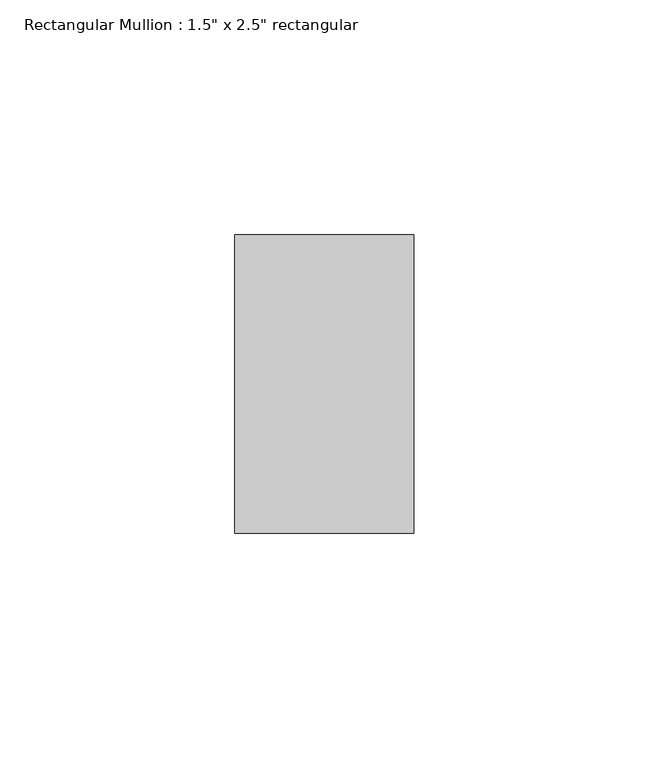
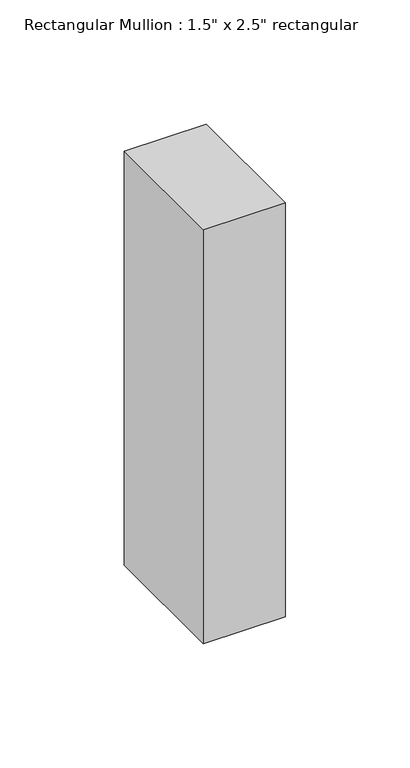
"""IFC4 building model written with IfcOpenShell, lengths in millimetres: member geometry."""

from ifc_helpers import new_model, si_unit, frame, origin, place, context, project, spatial, polyline, outline, extrude, source, transform, mapped, element, save


def member_56b223d9(model_context):
    return source(origin(), model_context, "Body", "SweptSolid", [
        extrude(outline(polyline([(19.05, 31.75), (19.05, -31.75), (-19.05, -31.75), (-19.05, 31.75), (19.05, 31.75)])), frame((0.0, 0.0, -203.2), z_axis=(0.0, 0.0, 1.0), x_axis=(1.0, 0.0, 0.0)), (0.0, 0.0, 1.0), 203.2),
    ])


if __name__ == "__main__":
    model = new_model("IFC4")
    model_context = context("Model", 3, world=origin())
    ifc_project = project(units=[si_unit("LENGTHUNIT", "METRE", prefix="MILLI")], contexts=[model_context])
    site = spatial("IfcSite", under=ifc_project)
    building = spatial("IfcBuilding", under=site)
    placement = place(None, origin())
    member_shape = member_56b223d9(model_context)
    element("IfcMember", 1, ObjectType="Rectangular Mullion : 1.5\" x 2.5\" rectangular", at=placement, inside=building, context=model_context, shape_type="MappedRepresentation", body=[
        mapped(member_shape, transform((0.0, 0.0, 0.0), x_axis=(1.0, 0.0, 0.0), y_axis=(0.0, 1.0, 0.0), z_axis=(0.0, 0.0, 1.0))),
    ])
    save(model, "model.ifc")

# Revit data of these elements
# Type "Rectangular Mullion : 1.5\" x 2.5\" rectangular"
#   built-in parameter 1007304 = 0.208333 (stored number, unit not read)
#   built-in parameter 1007301 = 0.0625 (stored number, unit not read)
#   built-in parameter 1007300 = 0.0625 (stored number, unit not read)
# Element 1 (IfcMember, "Rectangular Mullion : 1.5\" x 2.5\" rectangular")
#   Materials on its faces: "Aluminum"
# Materials
#   "Aluminum": class "Metal", colour RGB 247 247 247, transparency 0, Description = "Aluminum 6061", Cost = 0
